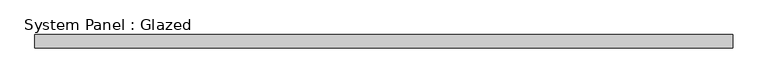
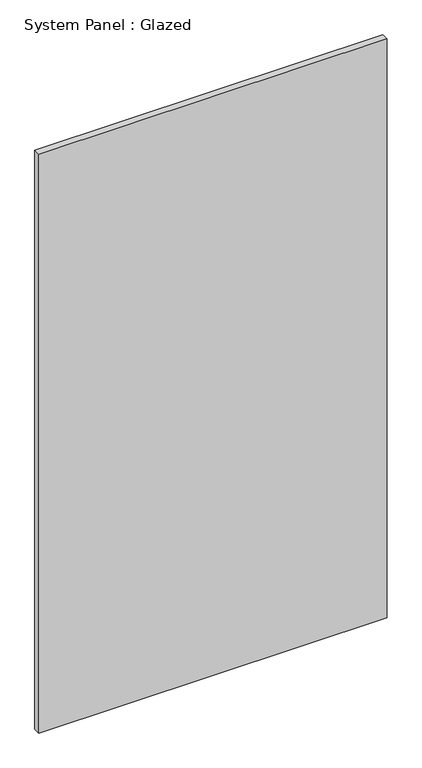
"""IFC4 building model written with IfcOpenShell, lengths in millimetres: plate geometry, System Panel : Glazed."""

from ifc_helpers import new_model, si_unit, origin, origin_with_axes, place, context, project, spatial, polyline, outline, extrude, source, transform, mapped, element, save


def system_panel_glazed_7a72b4ff(model_context):
    return source(origin(), model_context, "Body", "SweptSolid", [
        extrude(outline(polyline([(667.1592567, 19.05), (-667.1592567, 19.05), (-667.1592567, 44.45), (667.1592567, 44.45), (667.1592567, 19.05)])), origin_with_axes(), (0.0, 0.0, 1.0), 2343.15),
    ])


if __name__ == "__main__":
    model = new_model("IFC4")
    model_context = context("Model", 3, world=origin())
    ifc_project = project(units=[si_unit("LENGTHUNIT", "METRE", prefix="MILLI")], contexts=[model_context])
    site = spatial("IfcSite", under=ifc_project)
    building = spatial("IfcBuilding", under=site)
    placement = place(None, origin())
    system_panel_glazed_shape = system_panel_glazed_7a72b4ff(model_context)
    element("IfcPlate", 1, ObjectType="System Panel : Glazed", at=placement, inside=building, context=model_context, shape_type="MappedRepresentation", body=[
        mapped(system_panel_glazed_shape, transform((0.0, 0.0, 0.0), x_axis=(1.0, 0.0, 0.0), y_axis=(0.0, 1.0, 0.0), z_axis=(0.0, 0.0, 1.0))),
    ])
    save(model, "model.ifc")

# Revit data of these elements
# Type "System Panel : Glazed"
#   Construction Type Id = "GSP4R"
#   Analytic Construction = "1/8 in Pilkington single glazing"
#   Visual Light Transmittance = 0.9
#   Solar Heat Gain Coefficient = 0.86
#   Heat Transfer Coefficient (U) = 1.18115 BTU/(h·ft²·°F)
# Element 1 (IfcPlate, "System Panel : Glazed")
#   Materials on its faces: "Glass"
# Materials
#   "Glass": class "Glass", colour RGB 0 128 192, transparency 0.75, Description = "Soda Lime Glass", Cost = 0
